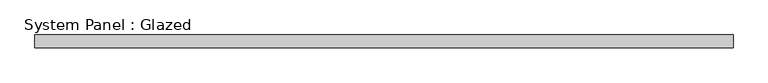
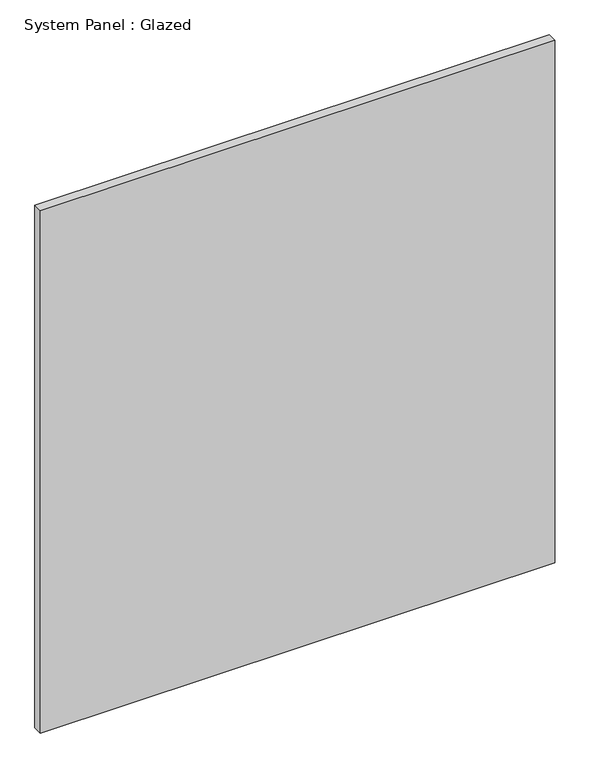
"""IFC4 building model written with IfcOpenShell, lengths in millimetres: plate geometry, System Panel : Glazed."""

from ifc_helpers import new_model, si_unit, origin, origin_with_axes, place, context, project, spatial, polyline, outline, extrude, source, transform, mapped, element, save


def system_panel_glazed_0767085a(model_context):
    return source(origin(), model_context, "Body", "SweptSolid", [
        extrude(outline(polyline([(692.15, 19.05), (-692.15, 19.05), (-692.15, 44.45), (692.15, 44.45), (692.15, 19.05)])), origin_with_axes(), (0.0, 0.0, 1.0), 1486.742764),
    ])


if __name__ == "__main__":
    model = new_model("IFC4")
    model_context = context("Model", 3, world=origin())
    ifc_project = project(units=[si_unit("LENGTHUNIT", "METRE", prefix="MILLI")], contexts=[model_context])
    site = spatial("IfcSite", under=ifc_project)
    building = spatial("IfcBuilding", under=site)
    placement = place(None, origin())
    system_panel_glazed_shape = system_panel_glazed_0767085a(model_context)
    element("IfcPlate", 1, ObjectType="System Panel : Glazed", at=placement, inside=building, context=model_context, shape_type="MappedRepresentation", body=[
        mapped(system_panel_glazed_shape, transform((0.0, 0.0, 0.0), x_axis=(1.0, 0.0, 0.0), y_axis=(0.0, 1.0, 0.0), z_axis=(0.0, 0.0, 1.0))),
    ])
    save(model, "model.ifc")

# Revit data of these elements
# Type "System Panel : Glazed"
#   Construction Type Id = "GSP4R"
#   Analytic Construction = "1/8 in Pilkington single glazing"
#   Visual Light Transmittance = 0.9
#   Solar Heat Gain Coefficient = 0.86
#   Heat Transfer Coefficient (U) = 1.18115 BTU/(h·ft²·°F)
#   Define Thermal Properties by = 1
# Element 1 (IfcPlate, "System Panel : Glazed")
#   Materials on its faces: "Glass"
# Materials
#   "Glass": class "Glass", colour RGB 0 128 192, transparency 0.75, Description = "Soda Lime Glass", Cost = 0
